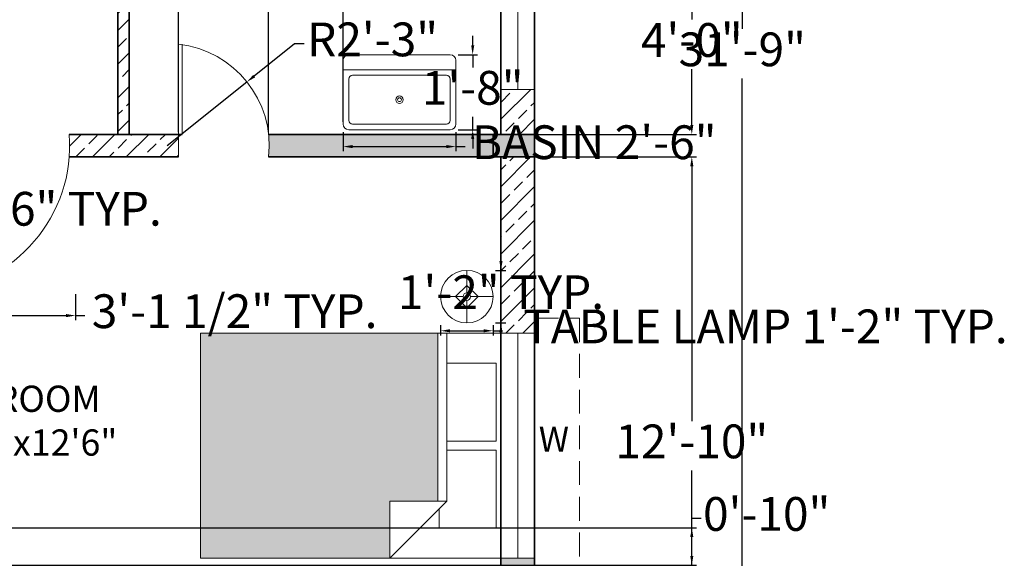
# Model space of a CAD drawing. Units: inches. Extents: x 9689 to 10369, y 10965 to 11626.
# Tile 10 of 11: x 10107 to 10369, y 11214 to 11357. Entities that reach past the tile are written whole.
import ezdxf

# ---------------------------------------------------------------- set-up
doc = ezdxf.new("R2010")
doc.units = ezdxf.units.IN
doc.linetypes.add('DASHED2', pattern=[9.525, 6.35, -3.175])
for name, color, linetype, lineweight in [('A-ANNO-DIMS', 2, 'Continuous', 18), ('A-ANNO-TEXT', 7, 'Continuous', 18), ('A-AREA-IDEN', 7, 'Continuous', 18), ('A-COLS', 7, 'Continuous', 35), ('A-DOOR', 4, 'Continuous', 18), ('A-FLOR-FIXT', 8, 'Continuous', 18), ('A-FURN', 8, 'Continuous', 18), ('A-GLAZ', 4, 'Continuous', 18), ('A-GLAZ-OVHD', 4, 'DASHED2', 13), ('A-WALL', 7, 'Continuous', 35), ('A-WALL-PATT', 252, 'Continuous', 13)]:
    doc.layers.add(name, color=color, linetype=linetype, lineweight=lineweight)
doc.layers.add('A-COLS-PATT', color=18, linetype='Continuous', lineweight=13, true_color=0x000000)
doc.layers.add('A-FURN-PATT', color=18, linetype='Continuous', lineweight=13, true_color=0x000000)
doc.styles.get("Standard").update_dxf_attribs({"font": 'arial.ttf'})
doc.dimstyles.new('ISO-25', dxfattribs={"dimtxt": 9, "dimasz": 2.5, "dimexe": 1.25, "dimexo": 0.625, "dimgap": 2, "dimtad": 0, "dimtih": 1, "dimtoh": 1, "dimdec": 1, "dimlunit": 4, "dimtxsty": 'Standard', "dimcen": 2.5, "dimadec": 0, "dimazin": 0, "dimtfac": 0.5, "dimtdec": 1, "dimtmove": 0, "dimatfit": 3, "dimfxl": 1, "dimarcsym": 0})

# ---------------------------------------------------------------- blocks, each defined once
blk = doc.blocks.new('Bed - Queen')
for p, q in [((0, -80.00003), (0, 0)), ((0, 0), (59.99999, 0)), ((59.99999, 0), (59.99999, -80.00003)), ((7.99999, -1.2), (28.79998, -1.2)), ((7.99999, -14.4), (7.99999, -1.2)), ((28.79998, -1.2), (28.79998, -14.4)), ((31.19999, -1.2), (51.99999, -1.2)), ((31.19999, -14.4), (31.19999, -1.2)), ((51.99999, -1.2), (51.99999, -16.4)), ((0, -14.4), (44.8, -14.4)), ((59.99999, -29.6), (44.8, -14.4)), ((44.8, -14.4), (44.8, -29.6)), ((44.8, -16.8), (0, -16.8)), ((51.99999, -16.4), (46.79936, -16.4)), ((44.8, -29.6), (59.99999, -29.6)), ((59.99999, -80.00003), (0, -80.00003))]:
    blk.add_line(p, q)
blk = doc.blocks.new('Lamp - Table')
for p, q in [((0, 7), (0, 1)), ((0, 3), (-3, 0)), ((3, 0), (0, 3)), ((-1, 0), (-7, 0)), ((-3, 0), (0, -3)), ((0, -3), (3, 0)), ((1, 0), (7, 0)), ((0, -1), (0, -7))]:
    blk.add_line(p, q)
for radius in [7, 1]:
    blk.add_circle((0, 0), radius)
blk = doc.blocks.new('*D22')
at = {"layer": 'A-ANNO-DIMS', "color": 0, "lineweight": -2, "transparency": 16777216}
for p, q in [((10244.68, 11538.63), (10300.66, 11538.63)), ((10299.41, 11536.13), (10299.41, 11354.73)), ((10299.41, 11160.13), (10299.41, 11341.53)), ((10244.68, 11157.63), (10300.66, 11157.63))]:
    blk.add_line(p, q, dxfattribs=at)
at = {"layer": 'A-ANNO-DIMS', "color": 0, "transparency": 16777216}
for points in [[(10298.99, 11536.13), (10299.83, 11536.13), (10299.41, 11538.63)], [(10298.99, 11160.13), (10299.83, 11160.13), (10299.41, 11157.63)]]:
    blk.add_solid(points, dxfattribs=at)
at = {"layer": 'Defpoints', "color": 0, "transparency": 16777216}
for p in [(10244.06, 11538.63), (10244.06, 11157.63), (10299.41, 11157.63)]:
    blk.add_point(p, dxfattribs=at)
at = {"layer": 'A-ANNO-DIMS', "color": 0, "transparency": 16777216, "insert": (10299.41, 11348.13), "char_height": 9, "attachment_point": 5}
blk.add_mtext('31\'-9"', dxfattribs=at)
blk = doc.blocks.new('Sink-single - 30 in top')
blk.add_line((-15, -3.999996), (15, -3.999996))
for points in [[(-13.5, 0), (13.5, 0)], [(-15, -18.499996), (-15, -1.5)], [(15, -1.5), (15, -18.499996)], [(-13.5, -17.499996), (-13.5, -6.499996)], [(-12.5, -5.499996), (12.5, -5.499996)], [(13.5, -6.499996), (13.5, -17.499996)], [(13.5, -19.999996), (-13.5, -19.999996)], [(12.5, -18.499996), (-12.5, -18.499996)]]:
    blk.add_lwpolyline(points)
for radius in [1, 0.5]:
    blk.add_circle((0, -11.999996), radius)
for centre, radius, start, end in [((-13.5, -1.5), 1.5, 90, 180), ((13.5, -1.5), 1.5, 0, 90), ((-12.5, -6.499996), 1, 90, 180), ((12.5, -6.499996), 1, 0, 90), ((-12.5, -17.499996), 1, 180, 270), ((12.5, -17.499996), 1, 270, 0), ((-13.5, -18.499996), 1.5, 180, 270), ((13.5, -18.499996), 1.5, 270, 0)]:
    blk.add_arc(centre, radius, start, end)
blk = doc.blocks.new('WINDOW-HOOD-68')
for p, q in [((12, 68), (0, 68)), ((0, 0), (0, 68)), ((12, 0), (0, 0))]:
    blk.add_line(p, q)
blk = doc.blocks.new('WINDOW-60')
for p, q in [((0, 60), (9, 60)), ((4.5, 60), (4.5, 0)), ((0, 0), (9, 0))]:
    blk.add_line(p, q)
blk = doc.blocks.new('WINDOW-24')
for p, q in [((0, 0), (0, 9)), ((24, 0), (24, 9)), ((0, 4.5), (24, 4.5))]:
    blk.add_line(p, q)
blk = doc.blocks.new('DOOR-SWING-36')
for p, q in [((0, 6), (0, 42)), ((1, 6), (1, 42)), ((0, 6), (0, 0))]:
    blk.add_line(p, q)
blk.add_arc((-3, 3), 39.12, 355.6013, 85.6013)
blk = doc.blocks.new('*D32')
at = {"layer": 'A-ANNO-DIMS', "color": 0, "lineweight": -2, "transparency": 16777216}
for p, q in [((10083.43, 11326.63), (10076.51, 11326.63)), ((10077.76, 11324.13), (10077.76, 11312.29)), ((10077.76, 11287.13), (10077.76, 11298.97)), ((10083.43, 11284.63), (10076.51, 11284.63))]:
    blk.add_line(p, q, dxfattribs=at)
at = {"layer": 'A-ANNO-DIMS', "color": 0, "transparency": 16777216}
for points in [[(10077.34, 11324.13), (10078.17, 11324.13), (10077.76, 11326.63)], [(10077.34, 11287.13), (10078.17, 11287.13), (10077.76, 11284.63)]]:
    blk.add_solid(points, dxfattribs=at)
at = {"layer": 'Defpoints', "color": 0, "transparency": 16777216}
for p in [(10084.06, 11326.63), (10077.76, 11284.63), (10084.06, 11284.63)]:
    blk.add_point(p, dxfattribs=at)
at = {"layer": 'A-ANNO-DIMS', "color": 0, "transparency": 16777216, "insert": (10077.76, 11305.63), "char_height": 9, "attachment_point": 5}
blk.add_mtext('DOOR SWING 3\'-6" TYP.', dxfattribs=at)
blk = doc.blocks.new('*D33')
at = {"layer": 'A-ANNO-DIMS', "color": 0, "lineweight": -2, "transparency": 16777216}
for p, q in [((10084.06, 11284.01), (10084.06, 11277.08)), ((10121.71, 11284.01), (10121.71, 11277.08)), ((10086.56, 11278.33), (10119.21, 11278.33)), ((10121.71, 11278.33), (10124.21, 11278.33))]:
    blk.add_line(p, q, dxfattribs=at)
at = {"layer": 'A-ANNO-DIMS', "color": 0, "transparency": 16777216}
for points in [[(10086.56, 11278.75), (10086.56, 11277.91), (10084.06, 11278.33)], [(10119.21, 11278.75), (10119.21, 11277.91), (10121.71, 11278.33)]]:
    blk.add_solid(points, dxfattribs=at)
at = {"layer": 'Defpoints', "color": 0, "transparency": 16777216}
for p in [(10084.06, 11284.63), (10121.71, 11284.63), (10121.71, 11278.33)]:
    blk.add_point(p, dxfattribs=at)
at = {"layer": 'A-ANNO-DIMS', "color": 0, "transparency": 16777216, "insert": (10164.13, 11278.33), "char_height": 9, "attachment_point": 5}
blk.add_mtext('3\'-1 1/2" TYP.', dxfattribs=at)
blk = doc.blocks.new('*D46')
at = {"layer": 'A-ANNO-DIMS', "color": 0, "lineweight": -2, "transparency": 16777216}
for p, q in [((10219.01, 11275.75), (10219.01, 11273.03)), ((10221.51, 11274.28), (10230.51, 11274.28)), ((10233.01, 11275.75), (10233.01, 11273.03)), ((10233.01, 11274.28), (10235.51, 11274.28))]:
    blk.add_line(p, q, dxfattribs=at)
at = {"layer": 'A-ANNO-DIMS', "color": 0, "transparency": 16777216}
for points in [[(10221.51, 11274.69), (10221.51, 11273.86), (10219.01, 11274.28)], [(10230.51, 11274.69), (10230.51, 11273.86), (10233.01, 11274.28)]]:
    blk.add_solid(points, dxfattribs=at)
at = {"layer": 'Defpoints', "color": 0, "transparency": 16777216}
for p in [(10219.01, 11276.38), (10233.01, 11276.38), (10233.01, 11274.28)]:
    blk.add_point(p, dxfattribs=at)
at = {"layer": 'A-ANNO-DIMS', "color": 0, "transparency": 16777216, "insert": (10305.58, 11274.28), "char_height": 9, "attachment_point": 5}
blk.add_mtext('TABLE LAMP 1\'-2" TYP.', dxfattribs=at)
blk = doc.blocks.new('*D47')
at = {"layer": 'A-ANNO-DIMS', "color": 0, "lineweight": -2, "transparency": 16777216}
for p, q in [((10235.11, 11292.88), (10235.11, 11295.38)), ((10233.63, 11290.38), (10236.36, 11290.38)), ((10235.11, 11290.38), (10235.11, 11289.9)), ((10235.11, 11276.38), (10235.11, 11276.85)), ((10233.63, 11276.38), (10236.36, 11276.38)), ((10235.11, 11273.88), (10235.11, 11271.38))]:
    blk.add_line(p, q, dxfattribs=at)
at = {"layer": 'A-ANNO-DIMS', "color": 0, "transparency": 16777216}
for points in [[(10234.69, 11292.88), (10235.53, 11292.88), (10235.11, 11290.38)], [(10234.69, 11273.88), (10235.53, 11273.88), (10235.11, 11276.38)]]:
    blk.add_solid(points, dxfattribs=at)
at = {"layer": 'Defpoints', "color": 0, "transparency": 16777216}
for p in [(10233.01, 11290.38), (10235.11, 11290.38), (10233.01, 11276.38)]:
    blk.add_point(p, dxfattribs=at)
at = {"layer": 'A-ANNO-DIMS', "color": 0, "transparency": 16777216, "insert": (10235.11, 11283.38), "char_height": 9, "attachment_point": 5}
blk.add_mtext('1\'-2" TYP.', dxfattribs=at)
blk = doc.blocks.new('*D64')
at = {"layer": 'A-ANNO-DIMS', "color": 0, "lineweight": -2, "transparency": 16777216}
for p, q in [((10193.07, 11327.25), (10193.07, 11322.12)), ((10223.07, 11327.25), (10223.07, 11322.12)), ((10195.57, 11323.37), (10220.57, 11323.37)), ((10223.07, 11323.37), (10225.57, 11323.37))]:
    blk.add_line(p, q, dxfattribs=at)
at = {"layer": 'A-ANNO-DIMS', "color": 0, "transparency": 16777216}
for points in [[(10195.57, 11323.79), (10195.57, 11322.96), (10193.07, 11323.37)], [(10220.57, 11323.79), (10220.57, 11322.96), (10223.07, 11323.37)]]:
    blk.add_solid(points, dxfattribs=at)
at = {"layer": 'Defpoints', "color": 0, "transparency": 16777216}
for p in [(10193.07, 11327.87), (10223.07, 11327.87), (10223.07, 11323.37)]:
    blk.add_point(p, dxfattribs=at)
at = {"layer": 'A-ANNO-DIMS', "color": 0, "transparency": 16777216, "insert": (10259.95, 11323.37), "char_height": 9, "attachment_point": 5}
blk.add_mtext('BASIN 2\'-6"', dxfattribs=at)
blk = doc.blocks.new('*D65')
at = {"layer": 'A-ANNO-DIMS', "color": 0, "lineweight": -2, "transparency": 16777216}
for p, q in [((10227.57, 11350.37), (10227.57, 11352.87)), ((10223.7, 11347.87), (10228.82, 11347.87)), ((10227.57, 11347.87), (10227.57, 11344.47)), ((10227.57, 11327.87), (10227.57, 11331.28)), ((10223.7, 11327.87), (10228.82, 11327.87)), ((10227.57, 11325.37), (10227.57, 11322.87))]:
    blk.add_line(p, q, dxfattribs=at)
at = {"layer": 'A-ANNO-DIMS', "color": 0, "transparency": 16777216}
for points in [[(10227.16, 11350.37), (10227.99, 11350.37), (10227.57, 11347.87)], [(10227.16, 11325.37), (10227.99, 11325.37), (10227.57, 11327.87)]]:
    blk.add_solid(points, dxfattribs=at)
at = {"layer": 'Defpoints', "color": 0, "transparency": 16777216}
for p in [(10223.07, 11347.87), (10227.57, 11347.87), (10223.07, 11327.87)]:
    blk.add_point(p, dxfattribs=at)
at = {"layer": 'A-ANNO-DIMS', "color": 0, "transparency": 16777216, "insert": (10227.57, 11337.87), "char_height": 9, "attachment_point": 5}
blk.add_mtext('1\'-8"', dxfattribs=at)
blk = doc.blocks.new('*D74')
at = {"layer": 'A-ANNO-DIMS', "color": 0, "lineweight": -2, "transparency": 16777216}
for p, q in [((10285.96, 11221.79), (10285.96, 11224.29)), ((10285.96, 11224.29), (10288.46, 11224.29)), ((10068.68, 11221.79), (10287.21, 11221.79)), ((10285.96, 11214.29), (10285.96, 11219.29)), ((10068.68, 11211.79), (10287.21, 11211.79))]:
    blk.add_line(p, q, dxfattribs=at)
at = {"layer": 'A-ANNO-DIMS', "color": 0, "transparency": 16777216}
for points in [[(10285.54, 11219.29), (10286.37, 11219.29), (10285.96, 11221.79)], [(10285.54, 11214.29), (10286.37, 11214.29), (10285.96, 11211.79)]]:
    blk.add_solid(points, dxfattribs=at)
at = {"layer": 'Defpoints', "color": 0, "transparency": 16777216}
for p in [(10068.06, 11221.79), (10285.96, 11221.79), (10068.06, 11211.79)]:
    blk.add_point(p, dxfattribs=at)
at = {"layer": 'A-ANNO-DIMS', "color": 0, "transparency": 16777216, "insert": (10305.92, 11224.29), "char_height": 9, "attachment_point": 5}
blk.add_mtext('0\'-10"', dxfattribs=at)
blk = doc.blocks.new('*D77')
at = {"layer": 'A-ANNO-DIMS', "color": 0, "lineweight": -2, "transparency": 16777216}
for p, q in [((10244.68, 11374.63), (10287.21, 11374.63)), ((10285.96, 11372.13), (10285.96, 11357.23)), ((10285.96, 11329.13), (10285.96, 11344.03)), ((10244.68, 11326.63), (10287.21, 11326.63))]:
    blk.add_line(p, q, dxfattribs=at)
at = {"layer": 'A-ANNO-DIMS', "color": 0, "transparency": 16777216}
for points in [[(10285.54, 11372.13), (10286.37, 11372.13), (10285.96, 11374.63)], [(10285.54, 11329.13), (10286.37, 11329.13), (10285.96, 11326.63)]]:
    blk.add_solid(points, dxfattribs=at)
at = {"layer": 'Defpoints', "color": 0, "transparency": 16777216}
for p in [(10244.06, 11374.63), (10285.96, 11374.63), (10244.06, 11326.63)]:
    blk.add_point(p, dxfattribs=at)
at = {"layer": 'A-ANNO-DIMS', "color": 0, "transparency": 16777216, "insert": (10285.96, 11350.63), "char_height": 9, "attachment_point": 5}
blk.add_mtext('4\'-0"', dxfattribs=at)
blk = doc.blocks.new('*D104')
at = {"layer": 'A-ANNO-DIMS', "color": 0, "lineweight": -2, "transparency": 16777216}
for p, q in [((10149.19, 11327.26), (10149.19, 11613.7)), ((10151.69, 11612.45), (10170.69, 11612.45)), ((10173.19, 11327.26), (10173.19, 11613.7)), ((10173.19, 11612.45), (10175.69, 11612.45))]:
    blk.add_line(p, q, dxfattribs=at)
at = {"layer": 'A-ANNO-DIMS', "color": 0, "transparency": 16777216}
for points in [[(10151.69, 11612.87), (10151.69, 11612.04), (10149.19, 11612.45)], [(10170.69, 11612.87), (10170.69, 11612.04), (10173.19, 11612.45)]]:
    blk.add_solid(points, dxfattribs=at)
at = {"layer": 'Defpoints', "color": 0, "transparency": 16777216}
for p in [(10173.19, 11612.45), (10149.19, 11326.63), (10173.19, 11326.63)]:
    blk.add_point(p, dxfattribs=at)
at = {"layer": 'A-ANNO-DIMS', "color": 0, "transparency": 16777216, "insert": (10189.73, 11612.45), "char_height": 9, "attachment_point": 5}
blk.add_mtext('2\'-0"', dxfattribs=at)
blk = doc.blocks.new('*D105')
at = {"layer": 'A-ANNO-DIMS', "color": 0, "lineweight": -2, "transparency": 16777216}
for p, q in [((10130.54, 11612.45), (10128.04, 11612.45)), ((10133.04, 11327.26), (10133.04, 11613.7)), ((10133.04, 11612.45), (10136.04, 11612.45)), ((10136.04, 11327.26), (10136.04, 11613.7)), ((10138.54, 11612.45), (10141.04, 11612.45))]:
    blk.add_line(p, q, dxfattribs=at)
at = {"layer": 'A-ANNO-DIMS', "color": 0, "transparency": 16777216}
for points in [[(10130.54, 11612.87), (10130.54, 11612.04), (10133.04, 11612.45)], [(10138.54, 11612.87), (10138.54, 11612.04), (10136.04, 11612.45)]]:
    blk.add_solid(points, dxfattribs=at)
at = {"layer": 'Defpoints', "color": 0, "transparency": 16777216}
for p in [(10136.04, 11612.45), (10133.04, 11326.63), (10136.04, 11326.63)]:
    blk.add_point(p, dxfattribs=at)
at = {"layer": 'A-ANNO-DIMS', "color": 0, "transparency": 16777216, "insert": (10155, 11612.45), "char_height": 9, "attachment_point": 5}
blk.add_mtext('0\'-3"', dxfattribs=at)
blk = doc.blocks.new('*D107')
at = {"layer": 'A-ANNO-DIMS', "color": 0, "lineweight": -2, "transparency": 16777216}
for p, q in [((10235.68, 11320.63), (10287.21, 11320.63)), ((10285.96, 11318.13), (10285.96, 11250.23)), ((10285.96, 11169.13), (10285.96, 11237.03)), ((10235.68, 11166.63), (10287.21, 11166.63))]:
    blk.add_line(p, q, dxfattribs=at)
at = {"layer": 'A-ANNO-DIMS', "color": 0, "transparency": 16777216}
for points in [[(10285.54, 11318.13), (10286.37, 11318.13), (10285.96, 11320.63)], [(10285.54, 11169.13), (10286.37, 11169.13), (10285.96, 11166.63)]]:
    blk.add_solid(points, dxfattribs=at)
at = {"layer": 'Defpoints', "color": 0, "transparency": 16777216}
for p in [(10235.06, 11320.63), (10285.96, 11320.63), (10235.06, 11166.63)]:
    blk.add_point(p, dxfattribs=at)
at = {"layer": 'A-ANNO-DIMS', "color": 0, "transparency": 16777216, "insert": (10285.96, 11243.63), "char_height": 9, "attachment_point": 5}
blk.add_mtext('12\'-10"', dxfattribs=at)
blk = doc.blocks.new('*D117')
at = {"layer": 'A-ANNO-DIMS', "color": 0, "lineweight": -2, "transparency": 16777216}
for p, q in [((10173.19, 11327.26), (10173.19, 11613.7)), ((10175.69, 11612.45), (10190.57, 11612.45)), ((10193.07, 11330), (10193.07, 11613.7)), ((10193.07, 11612.45), (10195.57, 11612.45))]:
    blk.add_line(p, q, dxfattribs=at)
at = {"layer": 'A-ANNO-DIMS', "color": 0, "transparency": 16777216}
for points in [[(10175.69, 11612.87), (10175.69, 11612.04), (10173.19, 11612.45)], [(10190.57, 11612.87), (10190.57, 11612.04), (10193.07, 11612.45)]]:
    blk.add_solid(points, dxfattribs=at)
at = {"layer": 'Defpoints', "color": 0, "transparency": 16777216}
for p in [(10193.07, 11612.45), (10193.07, 11329.37), (10173.19, 11326.63)]:
    blk.add_point(p, dxfattribs=at)
at = {"layer": 'A-ANNO-DIMS', "color": 0, "transparency": 16777216, "insert": (10209.11, 11612.45), "char_height": 9, "attachment_point": 5}
blk.add_mtext('1\'-8"', dxfattribs=at)
blk = doc.blocks.new('*D123')
at = {"layer": 'A-ANNO-DIMS', "color": 0, "lineweight": -2, "transparency": 16777216}
for p, q in [((10180.13, 11350.78), (10169.36, 11342.16)), ((10182.63, 11350.78), (10180.13, 11350.78)), ((10146.19, 11323.63), (10167.4, 11340.6))]:
    blk.add_line(p, q, dxfattribs=at)
at = {"layer": 'A-ANNO-DIMS', "color": 0, "transparency": 16777216}
blk.add_solid([(10169.1, 11342.49), (10169.62, 11341.84), (10167.4, 11340.6)], dxfattribs=at)
at = {"layer": 'Defpoints', "color": 0, "transparency": 16777216}
for p in [(10167.4, 11340.6), (10146.19, 11323.63)]:
    blk.add_point(p, dxfattribs=at)
at = {"layer": 'A-ANNO-DIMS', "color": 0, "transparency": 16777216, "insert": (10200.9, 11350.78), "char_height": 9, "attachment_point": 5}
blk.add_mtext('R2\'-3"', dxfattribs=at)

msp = doc.modelspace()

# ---------------------------------------------------------------- hatches: boundary and pattern name
at = {"layer": 'A-COLS-PATT'}
h = msp.add_hatch(color=256, dxfattribs=at)
h.dxf.hatch_style = 1
h.paths.add_polyline_path([(10244.06, 11326.63), (10235.06, 11326.63), (10233.06, 11326.63), (10233.06, 11320.63), (10235.06, 11320.63), (10244.06, 11320.63)])
at = {"layer": 'A-FURN-PATT'}
h = msp.add_hatch(color=256, dxfattribs=at)
h.dxf.hatch_style = 1
h.paths.add_polyline_path([(10184.09, 11495.26), (10168.89, 11495.26), (10168.89, 11508.06), (10124.09, 11508.06), (10124.09, 11444.86), (10184.09, 11444.86)])
h.paths.add_polyline_path([(10218.26, 11273.63), (10155.06, 11273.63), (10155.06, 11213.63), (10205.46, 11213.63), (10205.46, 11228.83), (10218.26, 11228.83)])
at = {"layer": 'A-WALL-PATT'}
h = msp.add_hatch(dxfattribs=at)
h.set_pattern_fill('ANSI33', color=256)
h.paths.add_polyline_path([(9843.06, 11538.63), (9811.06, 11538.63), (9811.06, 11529.63), (9843.06, 11529.63)])
h.paths.add_polyline_path([(9923.06, 11538.63), (9891.06, 11538.63), (9891.06, 11529.63), (9923.06, 11529.63)])
h.paths.add_polyline_path([(9929.06, 11527.63), (9923.06, 11527.63), (9923.06, 11380.63), (9929.06, 11380.63)])
h.paths.add_polyline_path([(9939.06, 11538.63), (9929.06, 11538.63), (9929.06, 11529.63), (9939.06, 11529.63, -0.071068)])
h.paths.add_polyline_path([(10035.06, 11538.63), (10013.06, 11538.63), (10013.06, 11529.63), (10022.06, 11529.63), (10022.06, 11507.38), (10022.06, 11502.38), (10022.06, 11482.38), (10022.06, 11478.38), (10022.06, 11456.13, -0.038405), (10026.06, 11456.13), (10026.06, 11502.38), (10026.06, 11529.63), (10035.06, 11529.63)])
h.paths.add_polyline_path([(10068.06, 11538.63), (10059.06, 11538.63), (10059.06, 11529.63), (10068.06, 11529.63)])
h.paths.add_polyline_path([(10074.06, 11527.63), (10068.06, 11527.63), (10068.06, 11431.13), (10026.06, 11431.13), (10022.06, 11431.13), (9980.06, 11431.13), (9976.06, 11431.13), (9976.06, 11425.13), (10068.06, 11425.13), (10068.06, 11380.63), (10074.06, 11380.63)])
h.paths.add_polyline_path([(10124.56, 11538.63), (10074.06, 11538.63), (10074.06, 11529.63), (10124.56, 11529.63)])
h.paths.add_polyline_path([(9980.06, 11507.38), (9980.06, 11529.63), (9989.06, 11529.63), (9989.06, 11538.63), (9976.06, 11538.63), (9976.06, 11529.63), (9976.06, 11503.38), (9976.06, 11483.38), (9976.06, 11478.38), (9980.06, 11478.38), (9997.06, 11478.38, -0.038405), (9997.06, 11482.38), (9980.06, 11482.38)])
h.paths.add_polyline_path([(10235.06, 11538.63), (10184.56, 11538.63), (10184.56, 11529.63), (10235.06, 11529.63)])
h.paths.add_polyline_path([(10244.06, 11527.63), (10235.06, 11527.63), (10235.06, 11485.13), (10244.06, 11485.13)])
h.paths.add_polyline_path([(10244.06, 11425.13), (10235.06, 11425.13), (10235.06, 11380.63), (10244.06, 11380.63)])
h.paths.add_polyline_path([(10233.06, 11380.63), (10120.06, 11380.63, -0.038405), (10120.06, 11374.63), (10133.04, 11374.63), (10133.04, 11326.63), (10120.06, 11326.63, -0.038405), (10120.06, 11320.63), (10149.19, 11320.63), (10149.19, 11326.63), (10136.04, 11326.63), (10136.04, 11374.63), (10233.06, 11374.63)])
h.paths.add_polyline_path([(10084.06, 11380.63), (10076.06, 11380.63), (10076.06, 11374.63), (10084.06, 11374.63)])
h.paths.add_polyline_path([(10244.06, 11374.63), (10235.06, 11374.63), (10235.06, 11362.63), (10244.06, 11362.63)])
h.paths.add_polyline_path([(10244.06, 11338.63), (10235.06, 11338.63), (10235.06, 11326.63), (10244.06, 11326.63)])
h.paths.add_polyline_path([(10233.06, 11326.63), (10173.19, 11326.63, -0.055385), (10173.19, 11320.63), (10233.06, 11320.63)], flags=0)
h.paths.add_polyline_path([(10244.06, 11320.63), (10235.06, 11320.63), (10235.06, 11273.63), (10244.06, 11273.63)])
h = msp.add_hatch(dxfattribs=at)
h.set_pattern_fill('ANSI36', color=256)
h.paths.add_polyline_path([(10233.06, 11326.63), (10173.19, 11326.63, -0.055385), (10173.19, 11320.63), (10233.06, 11320.63)])
h.paths.add_polyline_path([(10244.06, 11213.63), (10235.06, 11213.63), (10235.06, 11166.63), (10244.06, 11166.63)])
h.paths.add_polyline_path([(10233.06, 11166.63), (10184.56, 11166.63), (10184.56, 11157.63), (10233.06, 11157.63)])
h.paths.add_polyline_path([(10124.56, 11166.63), (10074.06, 11166.63), (10074.06, 11157.63), (10124.56, 11157.63)])
h.paths.add_polyline_path([(10074.06, 11318.63), (10068.06, 11318.63), (10068.06, 11168.63), (10074.06, 11168.63)])
h.paths.add_polyline_path([(10068.06, 11166.63), (10011.06, 11166.63), (10011.06, 11157.63), (10068.06, 11157.63)])
h.paths.add_polyline_path([(10011.06, 11318.63), (10005.06, 11318.63), (10005.06, 11168.63), (10011.06, 11168.63)])
h.paths.add_polyline_path([(10005.06, 11166.63), (9985.06, 11166.63), (9985.06, 11157.63), (10005.06, 11157.63)])
h.paths.add_polyline_path([(9937.06, 11166.63), (9898.06, 11166.63), (9898.06, 11157.63), (9937.06, 11157.63, -0.042779)])
h.paths.add_polyline_path([(9850.06, 11166.63), (9813.06, 11166.63), (9813.06, 11157.63), (9850.06, 11157.63)])
h.paths.add_polyline_path([(9811.06, 11213.63), (9802.06, 11213.63), (9802.06, 11166.63), (9811.06, 11166.63)])
h.paths.add_polyline_path([(9811.06, 11320.63), (9802.06, 11320.63), (9802.06, 11273.63), (9811.06, 11273.63)])
h.paths.add_polyline_path([(9811.06, 11439.11), (9802.06, 11439.11), (9802.06, 11326.63), (9811.06, 11326.63)])
h.paths.add_polyline_path([(9957.06, 11326.63), (9813.06, 11326.63), (9813.06, 11320.63), (9957.06, 11320.63)])
h.paths.add_polyline_path([(9811.06, 11527.63), (9802.06, 11527.63), (9802.06, 11499.11), (9811.06, 11499.11)])

# ---------------------------------------------------------------- linework, layer by layer
at = {"layer": 'A-COLS'}
for p, q in [((10233.06, 11326.63), (10233.06, 11320.63)), ((10235.06, 11326.63), (10244.06, 11326.63)), ((10235.06, 11320.63), (10244.06, 11320.63))]:
    msp.add_line(p, q, dxfattribs=at)
at = {"layer": 'A-DOOR'}
for p, q in [((10149.19, 11326.63), (10149.19, 11350.63)), ((10150.19, 11326.63), (10150.19, 11350.63)), ((10149.19, 11326.63), (10149.19, 11320.63)), ((10149.19, 11326.63), (10150.19, 11326.63))]:
    msp.add_line(p, q, dxfattribs=at)
msp.add_arc((10146.19, 11323.63), 27.17, 353.6598, 83.6598, dxfattribs=at)
at = {"layer": 'A-WALL'}
for p, q in [((10244.06, 11538.63), (10244.06, 11157.63)), ((10133.04, 11374.63), (10133.04, 11326.63)), ((10136.04, 11374.63), (10136.04, 11326.63)), ((10235.06, 11374.63), (10235.06, 11326.63)), ((10120.06, 11326.63), (10133.04, 11326.63)), ((10120.06, 11326.63), (10133.04, 11326.63)), ((10120.06, 11326.63), (10150.19, 11326.63)), ((10136.04, 11326.63), (10149.19, 11326.63)), ((10136.04, 11326.63), (10149.19, 11326.63)), ((10173.19, 11326.63), (10235.06, 11326.63)), ((10173.19, 11326.63), (10235.06, 11326.63)), ((10120.06, 11320.63), (10149.19, 11320.63)), ((10120.06, 11320.63), (10149.19, 11320.63)), ((10173.19, 11320.63), (10235.06, 11320.63)), ((10235.06, 11320.63), (10235.06, 11166.63))]:
    msp.add_line(p, q, dxfattribs=at)

# ---------------------------------------------------------------- block references
at = {"layer": 'A-DOOR', "extrusion": (0, 0, -1), "zscale": -1, "rotation": 180}
msp.add_blockref('DOOR-SWING-36', (-10084.06, 11326.63), dxfattribs=at)
at = {"layer": 'A-FLOR-FIXT'}
msp.add_blockref('Sink-single - 30 in top', (10208.07, 11347.87), dxfattribs=at)
at = {"layer": 'A-FURN'}
msp.add_blockref('Lamp - Table', (10226.01, 11283.38), dxfattribs=at)
at = {"layer": 'A-FURN', "rotation": 270}
msp.add_blockref('Bed - Queen', (10235.06, 11273.63), dxfattribs=at)
at = {"layer": 'A-GLAZ', "rotation": 270.0000000000104}
msp.add_blockref('WINDOW-24', (10235.06, 11362.63), dxfattribs=at)
at = {"layer": 'A-GLAZ'}
msp.add_blockref('WINDOW-60', (10235.06, 11213.63), dxfattribs=at)
at = {"layer": 'A-GLAZ-OVHD', "rotation": 180}
msp.add_blockref('WINDOW-HOOD-68', (10256.06, 11277.63), dxfattribs=at)

# ---------------------------------------------------------------- texts
at = {"layer": 'A-ANNO-TEXT', "insert": (10245.18, 11248.75), "char_height": 6.729, "attachment_point": 1}
msp.add_mtext_dynamic_manual_height_columns('{\\fArial|b1|i0|c0|p34;W}', width=31.3623, gutter_width=33.65, heights=[0], dxfattribs=at)
at = {"layer": 'A-AREA-IDEN', "insert": (10081.97, 11259.66), "char_height": 7, "attachment_point": 1}
msp.add_mtext_dynamic_manual_height_columns('{\\fArial|b1|i0|c0|p34;BEDROOM\\P13\'5"x12\'6"}', width=73.0838, gutter_width=12.5, heights=[0], dxfattribs=at)

# ---------------------------------------------------------------- dimensions: what is measured, and where the dimension line sits
at = {"layer": 'A-ANNO-DIMS'}
for base, p1, p2, picture, middle in [((10136.04, 11612.45), (10133.04, 11326.63), (10136.04, 11326.63), '*D105', (10155, 11612.45)), ((10173.19, 11612.45), (10149.19, 11326.63), (10173.19, 11326.63), '*D104', (10189.73, 11612.45)), ((10193.07, 11612.45), (10173.19, 11326.63), (10193.07, 11329.37), '*D117', (10209.11, 11612.45))]:
    dim = msp.add_linear_dim(base=base, p1=p1, p2=p2, dimstyle='ISO-25', override={"dimdec": 1, "dimlfac": 1, "dimrnd": 0, "dimzin": 1, "dimdsep": 46, "dimlunit": 4, "dimfrac": 2}, dxfattribs=at)
    dim.commit()
    dim.dimension.update_dxf_attribs({"geometry": picture, "text_midpoint": middle})
for base, p1, p2, override, picture, middle in [((10299.41, 11157.63), (10244.06, 11538.63), (10244.06, 11157.63), {"dimclrd": 0, "dimclre": 0, "dimclrt": 0}, '*D22', (10299.41, 11348.13)), ((10285.96, 11374.63), (10244.06, 11326.63), (10244.06, 11374.63), {"dimdec": 1, "dimlfac": 1, "dimrnd": 0, "dimzin": 1, "dimdsep": 46, "dimlunit": 4, "dimfrac": 2}, '*D77', (10285.96, 11350.63)), ((10227.57, 11347.87), (10223.07, 11327.87), (10223.07, 11347.87), {"dimdec": 1, "dimlfac": 1, "dimrnd": 0, "dimzin": 1, "dimdsep": 46, "dimlunit": 4, "dimfrac": 2}, '*D65', (10227.57, 11337.87)), ((10285.96, 11320.63), (10235.06, 11166.63), (10235.06, 11320.63), {"dimdec": 1, "dimlfac": 1, "dimrnd": 0, "dimzin": 1, "dimdsep": 46, "dimlunit": 4, "dimfrac": 2}, '*D107', (10285.96, 11243.63)), ((10285.96, 11221.79), (10068.06, 11211.79), (10068.06, 11221.79), {"dimdec": 1, "dimlfac": 1, "dimrnd": 0, "dimzin": 1, "dimdsep": 46, "dimlunit": 4, "dimfrac": 2}, '*D74', (10305.92, 11224.29))]:
    dim = msp.add_linear_dim(base=base, p1=p1, p2=p2, angle=90, dimstyle='ISO-25', override=override, dxfattribs=at)
    dim.commit()
    dim.dimension.update_dxf_attribs({"geometry": picture, "text_midpoint": middle})
dim = msp.add_radius_dim(center=(10146.19, 11323.63), mpoint=(10167.4, 11340.6), dimstyle='ISO-25', override={"dimdec": 1, "dimlfac": 1, "dimrnd": 0, "dimzin": 1, "dimdsep": 46, "dimlunit": 4, "dimfrac": 2}, dxfattribs=at)
dim.commit()
dim.dimension.update_dxf_attribs({"geometry": '*D123', "text_midpoint": (10200.9, 11350.78), "dimtype": 164})
for base, p1, p2, text, picture, middle in [((10223.07, 11323.37), (10193.07, 11327.87), (10223.07, 11327.87), 'BASIN <>', '*D64', (10259.95, 11323.37)), ((10233.01, 11274.28), (10219.01, 11276.38), (10233.01, 11276.38), 'TABLE LAMP <> TYP.', '*D46', (10305.58, 11274.28)), ((10121.7136, 11278.3301), (10084.0568, 11284.6301), (10121.7136, 11284.6301), '<> TYP.', '*D33', (10164.126, 11278.3301))]:
    dim = msp.add_linear_dim(base=base, p1=p1, p2=p2, text=text, dimstyle='ISO-25', override={"dimdec": 1, "dimlfac": 1, "dimrnd": 0, "dimzin": 1, "dimdsep": 46, "dimlunit": 4, "dimfrac": 2}, dxfattribs=at)
    dim.commit()
    dim.dimension.update_dxf_attribs({"geometry": picture, "text_midpoint": middle})
for base, p1, p2, angle, text, picture, middle in [((10077.76, 11284.63), (10084.06, 11326.63), (10084.06, 11284.63), 270, 'DOOR SWING <> TYP.', '*D32', (10077.76, 11305.63)), ((10235.11, 11290.38), (10233.01, 11276.38), (10233.01, 11290.38), 90, '<> TYP.', '*D47', (10235.11, 11283.38))]:
    dim = msp.add_linear_dim(base=base, p1=p1, p2=p2, angle=angle, text=text, dimstyle='ISO-25', override={"dimdec": 1, "dimlfac": 1, "dimrnd": 0, "dimzin": 1, "dimdsep": 46, "dimlunit": 4, "dimfrac": 2}, dxfattribs=at)
    dim.commit()
    dim.dimension.update_dxf_attribs({"geometry": picture, "text_midpoint": middle})

doc.saveas('drawing.dxf')
